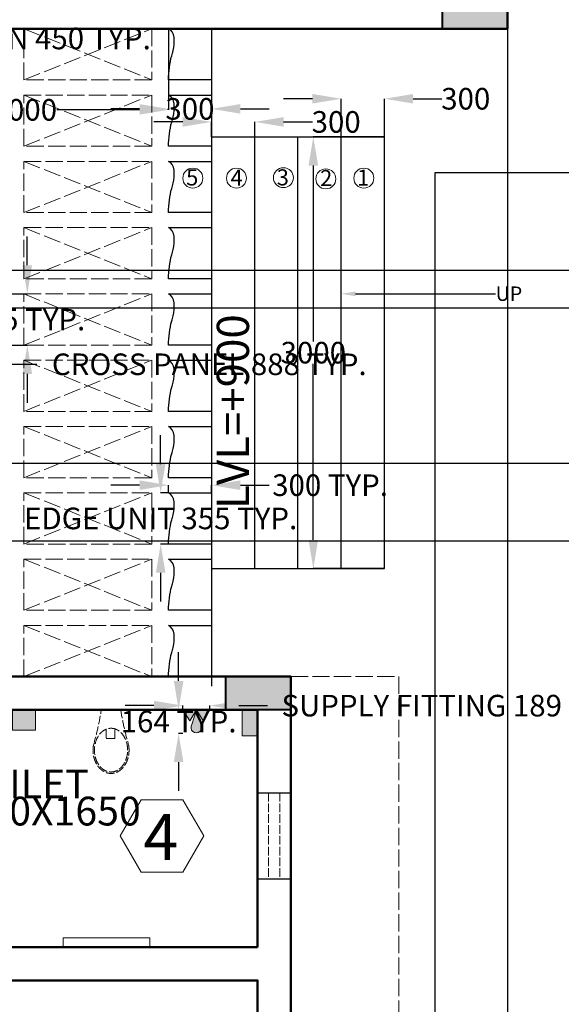
# Model space of a CAD drawing. Units: inches. Extents: x 22626 to 57351, y 2118 to 36234.
# Tile 7 of 10: x 45800 to 49561, y 16521 to 23360. Entities that reach past the tile are written whole.
import ezdxf
from ezdxf import colors
from ezdxf.entities.mleader import LeaderData, LeaderLine
from ezdxf.math import Vec2, Vec3

# ---------------------------------------------------------------- set-up
doc = ezdxf.new("R2010")
doc.units = ezdxf.units.IN
doc.header["$MEASUREMENT"] = 0
doc.linetypes.add('ACAD_ISO02W100', pattern=[15, 12, -3])
for name, color, linetype, lineweight in [('A-ANNO-DIMS', 130, 'Continuous', 18), ('A-ANNO-STRS', 130, 'Continuous', 15), ('A-ANNO-SYMB', 130, 'Continuous', 18), ('A-AREA-IDEN', 130, 'Continuous', 18), ('A-COLS', 7, 'Continuous', 40), ('A-FLOR-FIXT', 30, 'Continuous', 18), ('A-FLOR-FIXT-HIDN', 30, 'ACAD_ISO02W100', 18), ('A-GLAZ-VENT', 152, 'Continuous', 25), ('A-GLAZ-VENT-HIDN', 152, 'ACAD_ISO02W100', 18), ('A-ROOF', 80, 'Continuous', 25), ('A-ROOF-OVHD', 80, 'ACAD_ISO02W100', 18), ('A-WALL', 80, 'Continuous', 50), ('STAIRS', 82, 'Continuous', 25)]:
    doc.layers.add(name, color=color, linetype=linetype, lineweight=lineweight)
doc.styles.get("Standard").update_dxf_attribs({"font": 'arial.ttf'})
doc.dimstyles.get("Standard").update_dxf_attribs({"dimtxt": 150, "dimasz": 200, "dimexe": 0.18, "dimexo": 0.0625, "dimgap": 0.09, "dimtad": 0, "dimtih": 1, "dimtoh": 1, "dimdec": 0, "dimzin": 0, "dimdsep": 46, "dimtxsty": 'Standard', "dimcen": 0.09, "dimadec": 0, "dimazin": 0, "dimtfac": 1, "dimtdec": 0, "dimtofl": 0, "dimtmove": 0, "dimatfit": 3, "dimfxl": 1, "dimtolj": 1, "dimtzin": 0, "dimarcsym": 0})

# ---------------------------------------------------------------- blocks, each defined once
blk = doc.blocks.new('*D8')
at = {"layer": 'A-ANNO-DIMS', "color": 0, "lineweight": -2, "transparency": 16777216}
for p, q in [((48332.36654395866, 22546.86010836474), (47839.05636231795, 22546.86010836474)), ((47839.23636231794, 22346.86010836474), (47839.23636231794, 21123.587216141)), ((47839.23636231794, 19746.86010836474), (47839.23636231794, 20970.13300058848)), ((48332.36654395866, 19546.86010836473), (47839.05636231795, 19546.86010836473))]:
    blk.add_line(p, q, dxfattribs=at)
at = {"layer": 'A-ANNO-DIMS', "color": 0, "transparency": 16777216}
for points in [[(47805.90302898461, 22346.86010836474), (47872.56969565128, 22346.86010836474), (47839.23636231794, 22546.86010836474)], [(47805.90302898461, 19746.86010836474), (47872.56969565128, 19746.86010836474), (47839.23636231794, 19546.86010836473)]]:
    blk.add_solid(points, dxfattribs=at)
at = {"layer": 'Defpoints', "color": 0, "transparency": 16777216}
for p in [(48332.42904395866, 22546.86010836474), (47839.23636231794, 19546.86010836473), (48332.42904395866, 19546.86010836473)]:
    blk.add_point(p, dxfattribs=at)
at = {"layer": 'A-ANNO-DIMS', "color": 0, "transparency": 16777216, "insert": (47839.23636231794, 21046.86010836472), "char_height": 150, "attachment_point": 5}
blk.add_mtext('\\A1;3000', dxfattribs=at)
blk = doc.blocks.new('*D12')
at = {"layer": 'A-ANNO-DIMS', "color": 0, "lineweight": -2, "transparency": 16777216}
for p, q in [((44832.42904395864, 23296.79760836473), (44832.42904395864, 22733.54615739681)), ((46832.42904395864, 23296.79760836473), (46832.42904395864, 22733.54615739681)), ((45032.42904395865, 22733.72615739681), (45607.33904395865, 22733.72615739681)), ((46632.42904395865, 22733.72615739681), (46057.51904395864, 22733.72615739681))]:
    blk.add_line(p, q, dxfattribs=at)
at = {"layer": 'A-ANNO-DIMS', "color": 0, "transparency": 16777216}
for points in [[(45032.42904395865, 22767.05949073014), (45032.42904395865, 22700.39282406347), (44832.42904395864, 22733.72615739681)], [(46632.42904395865, 22767.05949073014), (46632.42904395865, 22700.39282406347), (46832.42904395864, 22733.72615739681)]]:
    blk.add_solid(points, dxfattribs=at)
at = {"layer": 'Defpoints', "color": 0, "transparency": 16777216}
for p in [(44832.42904395864, 23296.86010836473), (46832.42904395864, 23296.86010836473), (44832.42904395864, 22733.72615739681)]:
    blk.add_point(p, dxfattribs=at)
at = {"layer": 'A-ANNO-DIMS', "color": 0, "transparency": 16777216, "insert": (45832.42904395865, 22733.72615739681), "char_height": 150, "attachment_point": 5}
blk.add_mtext('\\A1;2000', dxfattribs=at)
blk = doc.blocks.new('*D13')
at = {"layer": 'A-ANNO-DIMS', "color": 0, "lineweight": -2, "transparency": 16777216}
for p, q in [((46632.22904395864, 22740.4612685317), (46432.22904395864, 22740.4612685317)), ((46832.22904395864, 22733.4086573968), (46832.22904395864, 22740.6412685317)), ((47132.42904395865, 22733.4086573968), (47132.42904395865, 22740.6412685317)), ((47332.42904395864, 22740.4612685317), (47532.42904395865, 22740.4612685317))]:
    blk.add_line(p, q, dxfattribs=at)
at = {"layer": 'A-ANNO-DIMS', "color": 0, "transparency": 16777216}
for points in [[(46632.22904395864, 22773.79460186503), (46632.22904395864, 22707.12793519837), (46832.22904395864, 22740.4612685317)], [(47332.42904395864, 22773.79460186503), (47332.42904395864, 22707.12793519837), (47132.42904395865, 22740.4612685317)]]:
    blk.add_solid(points, dxfattribs=at)
at = {"layer": 'Defpoints', "color": 0, "transparency": 16777216}
for p in [(46832.22904395864, 22733.34615739681), (47132.42904395865, 22740.4612685317), (47132.42904395865, 22733.34615739681)]:
    blk.add_point(p, dxfattribs=at)
at = {"layer": 'A-ANNO-DIMS', "color": 0, "transparency": 16777216, "insert": (46982.32904395864, 22740.4612685317), "char_height": 150, "attachment_point": 5}
blk.add_mtext('\\A1;300', dxfattribs=at)
blk = doc.blocks.new('*D14')
at = {"layer": 'A-ANNO-DIMS', "color": 0, "lineweight": -2, "transparency": 16777216}
for p, q in [((46932.42904395864, 22649.83293153023), (46732.42904395864, 22649.83293153023)), ((47132.42904395865, 22546.92260836473), (47132.42904395865, 22650.01293153023)), ((47432.42904395865, 22546.92260836473), (47432.42904395865, 22650.01293153023)), ((47632.42904395864, 22649.83293153023), (47832.42904395865, 22649.83293153023))]:
    blk.add_line(p, q, dxfattribs=at)
at = {"layer": 'A-ANNO-DIMS', "color": 0, "transparency": 16777216}
for points in [[(46932.42904395864, 22683.16626486356), (46932.42904395864, 22616.49959819689), (47132.42904395865, 22649.83293153023)], [(47632.42904395864, 22683.16626486356), (47632.42904395864, 22616.49959819689), (47432.42904395865, 22649.83293153023)]]:
    blk.add_solid(points, dxfattribs=at)
at = {"layer": 'Defpoints', "color": 0, "transparency": 16777216}
for p in [(47432.42904395865, 22649.83293153023), (47132.42904395865, 22546.86010836473), (47432.42904395865, 22546.86010836473)]:
    blk.add_point(p, dxfattribs=at)
at = {"layer": 'A-ANNO-DIMS', "color": 0, "transparency": 16777216, "insert": (47997.91808897911, 22649.83293153023), "char_height": 150, "attachment_point": 5}
blk.add_mtext('\\A1;300', dxfattribs=at)
blk = doc.blocks.new('*D15')
at = {"layer": 'A-ANNO-DIMS', "color": 0, "lineweight": -2, "transparency": 16777216}
for p, q in [((47832.42904395865, 22810.73997100012), (47632.42904395864, 22810.73997100012)), ((48032.42904395864, 22546.92260836473), (48032.42904395864, 22810.91997100012)), ((48332.42904395865, 22546.92260836473), (48332.42904395865, 22810.91997100012)), ((48532.42904395864, 22810.73997100012), (48732.42904395865, 22810.73997100012))]:
    blk.add_line(p, q, dxfattribs=at)
at = {"layer": 'A-ANNO-DIMS', "color": 0, "transparency": 16777216}
for points in [[(47832.42904395865, 22844.07330433345), (47832.42904395865, 22777.40663766679), (48032.42904395864, 22810.73997100012)], [(48532.42904395864, 22844.07330433345), (48532.42904395864, 22777.40663766679), (48332.42904395865, 22810.73997100012)]]:
    blk.add_solid(points, dxfattribs=at)
at = {"layer": 'Defpoints', "color": 0, "transparency": 16777216}
for p in [(48332.42904395865, 22810.73997100012), (48032.42904395864, 22546.86010836473), (48332.42904395865, 22546.86010836473)]:
    blk.add_point(p, dxfattribs=at)
at = {"layer": 'A-ANNO-DIMS', "color": 0, "transparency": 16777216, "insert": (48897.91808897911, 22810.73997100012), "char_height": 150, "attachment_point": 5}
blk.add_mtext('\\A1;300', dxfattribs=at)
blk = doc.blocks.new('WC')
at = {"ltscale": 5}
for p, q in [((307.4540408789253, 157.9229967620813), (242.2174300020561, 157.9229967620813)), ((242.2174300020561, 157.9229967620813), (242.2174300020561, 97.87988847275483)), ((307.4540408789253, 157.9229967620813), (307.4540408789253, 157.9229967620813)), ((242.2174300020561, 97.87988847275483), (310.0842174796853, 99.70460823710528))]:
    blk.add_line(p, q, dxfattribs=at)
for centre, start, end in [((780.732508801062, 2286.288249576111), 254.000576969056, 260.8285458946419), ((780.732508801062, -2036.267674000785), 99.17145410535805, 105.999423030944)]:
    blk.add_arc(centre, 2121.236142909723, start, end, dxfattribs=at)
blk.add_ellipse((161.9027973060947, 125.0102877876634), major_axis=(151.9040759523413, 0), ratio=0.7571275708385353, start_param=-1.570796326794896, end_param=4.712388980384689, dxfattribs=at)
for points, knots in [([(196.0611207178517, 247.2193096078299), (189.9898489161132, 248.2266596507652), (183.8456655129121, 248.9650412442752), (168.6182293347155, 250.1102459839712), (159.4964975931143, 250.2034131541222), (141.3581357193834, 249.212698022955), (132.3417047420516, 248.1288311957833), (114.6613914742556, 244.8098406800164), (105.9976853845146, 242.5747636017513), (89.26201623554518, 237.0062334978611), (81.19018288652298, 233.6728365616509), (65.86452451616788, 225.9859897466813), (58.61077128878969, 221.6325587335632), (45.13156838521536, 212.0080719868456), (38.90616664764093, 206.7369257869286), (27.67640637096338, 195.4043234284545), (22.67220516936504, 189.3426231032536), (14.05759261523781, 176.5860631599644), (10.44766267286468, 169.8909471035294), (4.765577569938614, 156.0629077761186), (2.69424158098991, 148.9301527436837), (0.1846293913040426, 134.463597005164), (-0.2530317139462568, 127.1307025187488), (0.5271766823570943, 112.5265070110981), (1.744832412616233, 105.2563518462193), (5.77749157987273, 91.03263116568269), (8.591685077881264, 84.07962673572185), (15.69573821845551, 70.70922901844096), (19.98490811580268, 64.29173781119243), (29.87879523489392, 52.16900764399179), (35.483208879421, 46.46348057011346), (47.82439502190391, 35.90657261581146), (54.56108629030495, 31.05501885116246), (68.96556532807881, 22.32099587028279), (76.63330319123634, 18.43849746629348), (92.68186228567357, 11.73355477496807), (101.0625846676266, 8.91115468616772), (118.3043576900527, 4.392898517646244), (127.1652540279829, 2.697098106120392), (144.6597339432555, 0.5298149587142689), (153.2812269904534, -0.000476238605188), (161.9027973060947, -0.000476238605188)], [1.35503494441986, 1.35503494441986, 1.35503494441986, 1.35503494441986, 1.471789532681877, 1.471789532681877, 1.642812487519809, 1.642812487519809, 1.813835442357741, 1.813835442357741, 1.984858397195673, 1.984858397195673, 2.155881352033606, 2.155881352033606, 2.326904306871538, 2.326904306871538, 2.49792726170947, 2.49792726170947, 2.668950216547402, 2.668950216547402, 2.839973171385334, 2.839973171385334, 3.010996126223266, 3.010996126223266, 3.182019081061198, 3.182019081061198, 3.35304203589913, 3.35304203589913, 3.524064990737062, 3.524064990737062, 3.695087945574994, 3.695087945574994, 3.866110900412926, 3.866110900412926, 4.037133855250859, 4.037133855250859, 4.208156810088791, 4.208156810088791, 4.379179764926723, 4.379179764926723, 4.550202719764655, 4.550202719764655, 4.712388980384689, 4.712388980384689, 4.712388980384689, 4.712388980384689]), ([(161.9027973060947, -0.000476238605188), (167.8851873344465, -0.000476238605188), (173.8675648995122, 0.254611844480678), (185.2699231324077, 1.230286525809788), (190.6953945214336, 1.911114408936555), (196.0639028232108, 2.802063691000512)], [-1.570796326794896, -1.570796326794896, -1.570796326794896, -1.570796326794896, -1.458257493061962, -1.458257493061962, -1.355016516099114, -1.355016516099114, -1.355016516099114, -1.355016516099114])]:
    blk.add_open_spline(points, degree=3, knots=knots, dxfattribs=at)
blk = doc.blocks.new('COL-RECTANGULAR')
h = blk.add_hatch(color=256)
h.dxf.hatch_style = 1
h.paths.add_polyline_path([(4.39586474386e-05, 0.0001083647293854), (450.0000439586474, 0.0001083647293854), (450.0000439586474, 230.0001083647294), (4.39586474386e-05, 230.0001083647294)])
blk.add_lwpolyline([(4.39586474386e-05, 0.0001083647293854), (4.39586474386e-05, 230.0001083647294), (450.0000439586474, 230.0001083647294), (450.0000439586474, 0.0001083647293854)], close=True)
blk = doc.blocks.new('CANOPY-CROSSED-PANEL')
at = {"ltscale": 10}
for p, q in [((4.39586510765e-05, -7.7958175098e-06), (887.5000439586511, 355.3241083647299)), ((4.39586510765e-05, 355.3241083647299), (887.5000439586511, -7.7958175098e-06))]:
    blk.add_line(p, q, dxfattribs=at)
blk.add_lwpolyline([(4.39586510765e-05, 355.3241083647299), (887.5000439586511, 355.3241083647299), (887.5000439586511, -7.7958175098e-06), (4.39586510765e-05, -7.7958175098e-06)], close=True, dxfattribs=at)
blk = doc.blocks.new('CANOPY-EDGE-UNIT')
blk.add_lwpolyline([(4.39586510765e-05, 355.3241083647299), (300.0000439586511, 355.3241083647299), (300.0000439586511, -7.7958211477e-06), (4.39586510765e-05, -7.7958211477e-06)])
blk.add_open_spline([(4.39586510765e-05, -7.7958211477e-06), (4.431511672410124, 57.50918677931622), (9.829222033331462, 127.5577565662788), (45.33431013918743, 237.7808474231315), (48.5081452225204, 340.4779943810172), (4.39586510765e-05, 355.3241083647299)], degree=3, knots=[0, 0, 0, 0, 169.2538425934583, 206.1581577034206, 361.8230239706648, 361.8230239706648, 361.8230239706648, 361.8230239706648])
blk = doc.blocks.new('BATH-SUPPLY-FITTING')
h = blk.add_hatch(color=256)
h.dxf.hatch_style = 1
h.paths.add_polyline_path([(161.0140439586466, 189.3806798614205), (84.84003036547074, 140.983449503361), (161.0140439586466, 94.69046873241678)])
h = blk.add_hatch(color=256)
h.dxf.hatch_style = 1
h.paths.add_polyline_path([(161.0140439586466, 94.69046873241678), (58.24591656582924, 125.2086534748123, 1.90856376211952), (58.24591656582924, 64.17228399002124)])
h = blk.add_hatch(color=256)
h.dxf.hatch_style = 1
h.paths.add_polyline_path([(161.0140439586466, 94.69046873241678), (84.84003036547074, 48.39748796147251), (161.0140439586466, 0.000257603413047)])
for p, q in [((161.0140439586466, 189.3806798614205), (84.84003036547074, 140.983449503361)), ((84.84003036547074, 140.983449503361), (161.0140439586466, 94.69046873241678)), ((161.0140439586466, 94.69046873241678), (58.24591656582924, 125.2086534748123)), ((161.0140439586466, 94.69046873241678), (58.24591656582924, 64.17228399002124)), ((84.84003036547074, 48.39748796147251), (161.0140439586466, 94.69046873241678)), ((161.0140439586466, 0.000257603413047), (84.84003036547074, 48.39748796147251))]:
    blk.add_line(p, q)
blk.add_arc((37.11803136635718, 94.69046873241678), 37.11801628553248, 55.30495923588778, 304.6950407641123)
blk = doc.blocks.new('BATH-WALL-ACCESSORY')
h = blk.add_hatch(color=256)
h.dxf.hatch_style = 1
h.paths.add_polyline_path([(142.8430439586445, 231.1050653827879), (71.42162994010141, 231.1050653827879), (71.42162994010141, 158.5160872540764), (81.4216299401014, 158.5160872540764), (81.42162994010869, 221.1050653827879), (142.8430439586445, 221.1050653827879)])
h = blk.add_hatch(color=256)
h.dxf.hatch_style = 1
h.paths.add_polyline_path([(142.8430439586445, 158.5160872540764), (0.0002159215582651, 158.5160872540764), (0.0002159215582651, -1.22242890939e-05), (142.8430439586445, -1.22242854559e-05)])
for p, q in [((71.42162994010141, 158.5160872540764), (71.42162994010141, 231.1050653827879)), ((71.42162994010141, 231.1050653827879), (142.8430439586445, 231.1050653827879)), ((81.42162994010869, 221.1050653827879), (142.8430439586445, 221.1050653827879)), ((81.4216299401014, 158.5160872540764), (81.42162994010869, 221.1050653827879)), ((142.8430439586445, 158.5160872540764), (0.0002159215582651, 158.5160872540764)), ((0.0002159215582651, 158.5160872540764), (0.0002159215582651, -1.22242890939e-05)), ((142.8430439586445, 158.5160872540764), (142.8430439586445, 158.5160872540764)), ((0.0002159215582651, -1.22242890939e-05), (142.8430439586445, -1.22242854559e-05))]:
    blk.add_line(p, q)
blk = doc.blocks.new('BATH-WALL-BOX')
h = blk.add_hatch(color=256)
h.dxf.hatch_style = 1
h.paths.add_polyline_path([(182.0210439586444, 106.8341357510071), (0.000183795193152, 106.8341357510071), (0.000183795193152, 0.0001083647293854), (182.0210439586444, 0.0001083647293854)])
for p, q in [((0.000183795193152, 0.0001083647293854), (0.000183795193152, 106.8341357510071)), ((0.000183795193152, 106.8341357510071), (182.0210439586444, 106.8341357510071)), ((182.0210439586444, 0.0001083647293854), (0.000183795193152, 0.0001083647293854))]:
    blk.add_line(p, q)
blk = doc.blocks.new('*D50')
at = {"layer": 'A-ANNO-DIMS', "color": 0, "lineweight": -2, "transparency": 16777216}
for p, q in [((44832.42904395864, 21099.39532160887), (44832.42904395864, 20966.15282160887)), ((45719.92904395863, 21099.39532160887), (45719.92904395863, 20966.15282160887)), ((45032.42904395864, 20966.33282160887), (45519.92904395864, 20966.33282160887)), ((45719.92904395863, 20966.33282160887), (45919.92904395864, 20966.33282160887))]:
    blk.add_line(p, q, dxfattribs=at)
at = {"layer": 'A-ANNO-DIMS', "color": 0, "transparency": 16777216}
for points in [[(45032.42904395864, 20999.6661549422), (45032.42904395864, 20932.99948827554), (44832.42904395864, 20966.33282160887)], [(45519.92904395864, 20999.6661549422), (45519.92904395864, 20932.99948827554), (45719.92904395863, 20966.33282160887)]]:
    blk.add_solid(points, dxfattribs=at)
at = {"layer": 'Defpoints', "color": 0, "transparency": 16777216}
for p in [(44832.42904395864, 21099.45782160887), (45719.92904395863, 21099.45782160887), (45719.92904395863, 20966.33282160887)]:
    blk.add_point(p, dxfattribs=at)
at = {"layer": 'A-ANNO-DIMS', "color": 0, "transparency": 16777216, "insert": (47116.89830726013, 20966.33282160887), "char_height": 150, "attachment_point": 5}
blk.add_mtext('\\A1;CROSS PANEL 888 TYP.', dxfattribs=at)
blk = doc.blocks.new('*D51')
at = {"layer": 'A-ANNO-DIMS', "color": 0, "lineweight": -2, "transparency": 16777216}
for p, q in [((45853.05404395866, 21654.78193776943), (45853.05404395866, 21854.78193776943)), ((45719.99154395865, 21454.78193776943), (45853.23404395866, 21454.78193776943)), ((45719.99154395865, 21099.45782160888), (45853.23404395866, 21099.45782160888)), ((45853.05404395866, 20899.45782160888), (45853.05404395866, 20699.45782160888))]:
    blk.add_line(p, q, dxfattribs=at)
at = {"layer": 'A-ANNO-DIMS', "color": 0, "transparency": 16777216}
for points in [[(45819.72071062534, 21654.78193776943), (45886.387377292, 21654.78193776943), (45853.05404395866, 21454.78193776943)], [(45819.72071062534, 20899.45782160888), (45886.387377292, 20899.45782160888), (45853.05404395866, 21099.45782160888)]]:
    blk.add_solid(points, dxfattribs=at)
at = {"layer": 'Defpoints', "color": 0, "transparency": 16777216}
for p in [(45719.92904395865, 21454.78193776943), (45853.05404395866, 21454.78193776943), (45719.92904395865, 21099.45782160888)]:
    blk.add_point(p, dxfattribs=at)
at = {"layer": 'A-ANNO-DIMS', "color": 0, "transparency": 16777216, "insert": (45853.05404395866, 21277.11987968914), "char_height": 150, "attachment_point": 5}
blk.add_mtext('\\A1;355 TYP.', dxfattribs=at)
blk = doc.blocks.new('*D54')
at = {"layer": 'A-ANNO-DIMS', "color": 0, "lineweight": -2, "transparency": 16777216}
for p, q in [((46779.13042653459, 20273.22330982295), (46779.13042653459, 20473.22330982295)), ((46832.36654395865, 20073.22330982295), (46778.95042653458, 20073.22330982295)), ((46832.36654395865, 19717.8991936624), (46778.95042653458, 19717.8991936624)), ((46779.13042653459, 19517.89919366239), (46779.13042653459, 19317.8991936624))]:
    blk.add_line(p, q, dxfattribs=at)
at = {"layer": 'A-ANNO-DIMS', "color": 0, "transparency": 16777216}
for points in [[(46745.79709320125, 20273.22330982295), (46812.46375986792, 20273.22330982295), (46779.13042653459, 20073.22330982295)], [(46745.79709320125, 19517.89919366239), (46812.46375986792, 19517.89919366239), (46779.13042653459, 19717.8991936624)]]:
    blk.add_solid(points, dxfattribs=at)
at = {"layer": 'Defpoints', "color": 0, "transparency": 16777216}
for p in [(46779.13042653459, 20073.22330982295), (46832.42904395865, 20073.22330982295), (46832.42904395865, 19717.8991936624)]:
    blk.add_point(p, dxfattribs=at)
at = {"layer": 'A-ANNO-DIMS', "color": 0, "transparency": 16777216, "insert": (46779.13042653459, 19895.56125174265), "char_height": 150, "attachment_point": 5}
blk.add_mtext('\\A1;EDGE UNIT 355 TYP.', dxfattribs=at)
blk = doc.blocks.new('*D55')
at = {"layer": 'A-ANNO-DIMS', "color": 0, "lineweight": -2, "transparency": 16777216}
for p, q in [((46632.42904395864, 20126.52192724702), (46432.42904395863, 20126.52192724702)), ((46832.42904395863, 20073.28580982294), (46832.42904395863, 20126.70192724702)), ((47132.42904395864, 20073.28580982294), (47132.42904395864, 20126.70192724702)), ((47332.42904395864, 20126.52192724702), (47532.42904395864, 20126.52192724702))]:
    blk.add_line(p, q, dxfattribs=at)
at = {"layer": 'A-ANNO-DIMS', "color": 0, "transparency": 16777216}
for points in [[(46632.42904395864, 20159.85526058035), (46632.42904395864, 20093.18859391369), (46832.42904395863, 20126.52192724702)], [(47332.42904395864, 20159.85526058035), (47332.42904395864, 20093.18859391369), (47132.42904395864, 20126.52192724702)]]:
    blk.add_solid(points, dxfattribs=at)
at = {"layer": 'Defpoints', "color": 0, "transparency": 16777216}
for p in [(47132.42904395864, 20126.52192724702), (46832.42904395863, 20073.22330982294), (47132.42904395864, 20073.22330982294)]:
    blk.add_point(p, dxfattribs=at)
at = {"layer": 'A-ANNO-DIMS', "color": 0, "transparency": 16777216, "insert": (47955.81372335837, 20126.52192724702), "char_height": 150, "attachment_point": 5}
blk.add_mtext('\\A1;300 TYP.', dxfattribs=at)
blk = doc.blocks.new('*D56')
at = {"layer": 'A-ANNO-DIMS', "color": 0, "lineweight": -2, "transparency": 16777216}
for p, q in [((44302.42904395863, 23296.79760836473), (44302.42904395863, 23229.18010836473)), ((44752.42904395862, 23296.79760836473), (44752.42904395862, 23229.18010836473)), ((44502.42904395863, 23229.36010836473), (44552.42904395862, 23229.36010836473)), ((44752.42904395862, 23229.36010836473), (44952.42904395862, 23229.36010836473))]:
    blk.add_line(p, q, dxfattribs=at)
at = {"layer": 'A-ANNO-DIMS', "color": 0, "transparency": 16777216}
for points in [[(44502.42904395863, 23262.69344169806), (44502.42904395863, 23196.0267750314), (44302.42904395863, 23229.36010836473)], [(44552.42904395862, 23262.69344169806), (44552.42904395862, 23196.0267750314), (44752.42904395862, 23229.36010836473)]]:
    blk.add_solid(points, dxfattribs=at)
at = {"layer": 'Defpoints', "color": 0, "transparency": 16777216}
for p in [(44302.42904395863, 23296.86010836473), (44752.42904395862, 23296.86010836473), (44752.42904395862, 23229.36010836473)]:
    blk.add_point(p, dxfattribs=at)
at = {"layer": 'A-ANNO-DIMS', "color": 0, "transparency": 16777216, "insert": (45858.14660193952, 23229.36010836473), "char_height": 150, "attachment_point": 5}
blk.add_mtext('\\A1;COLUMN 450 TYP.', dxfattribs=at)
blk = doc.blocks.new('*D66')
at = {"layer": 'A-ANNO-DIMS', "color": 0, "lineweight": -2, "transparency": 16777216}
for p, q in [((46732.21802730284, 18595.26717170344), (46532.21802730284, 18595.26717170344)), ((46932.21802730284, 18566.92260836473), (46932.21802730284, 18595.44717170344)), ((47121.59844956086, 18566.92260836473), (47121.59844956086, 18595.44717170344)), ((47321.59844956085, 18595.26717170344), (47521.59844956086, 18595.26717170344))]:
    blk.add_line(p, q, dxfattribs=at)
at = {"layer": 'A-ANNO-DIMS', "color": 0, "transparency": 16777216}
for points in [[(46732.21802730284, 18628.60050503677), (46732.21802730284, 18561.93383837011), (46932.21802730284, 18595.26717170344)], [(47321.59844956085, 18628.60050503677), (47321.59844956085, 18561.93383837011), (47121.59844956086, 18595.26717170344)]]:
    blk.add_solid(points, dxfattribs=at)
at = {"layer": 'Defpoints', "color": 0, "transparency": 16777216}
for p in [(46932.21802730284, 18566.86010836473), (47121.59844956086, 18595.26717170344), (47121.59844956086, 18566.86010836473)]:
    blk.add_point(p, dxfattribs=at)
at = {"layer": 'A-ANNO-DIMS', "color": 0, "transparency": 16777216, "insert": (48823.75188748719, 18595.26717170344), "char_height": 150, "attachment_point": 5}
blk.add_mtext('\\A1;SUPPLY FITTING 189 TYP.', dxfattribs=at)
blk = doc.blocks.new('*D67')
at = {"layer": 'A-ANNO-DIMS', "color": 0, "lineweight": -2, "transparency": 16777216}
for p, q in [((46903.81096396418, 18766.86010836474), (46903.81096396418, 18966.86010836474)), ((46932.15552730285, 18566.86010836474), (46903.63096396417, 18566.86010836474)), ((46932.15552730286, 18402.73068226325), (46903.63096396417, 18402.73068226325)), ((46903.81096396418, 18202.73068226325), (46903.81096396418, 18002.73068226325))]:
    blk.add_line(p, q, dxfattribs=at)
at = {"layer": 'A-ANNO-DIMS', "color": 0, "transparency": 16777216}
for points in [[(46870.47763063084, 18766.86010836474), (46937.14429729751, 18766.86010836474), (46903.81096396418, 18566.86010836474)], [(46870.47763063084, 18202.73068226325), (46937.14429729751, 18202.73068226325), (46903.81096396418, 18402.73068226325)]]:
    blk.add_solid(points, dxfattribs=at)
at = {"layer": 'Defpoints', "color": 0, "transparency": 16777216}
for p in [(46903.81096396418, 18566.86010836474), (46932.21802730286, 18566.86010836474), (46932.21802730286, 18402.73068226325)]:
    blk.add_point(p, dxfattribs=at)
at = {"layer": 'A-ANNO-DIMS', "color": 0, "transparency": 16777216, "insert": (46903.81096396418, 18484.79539531398), "char_height": 150, "attachment_point": 5}
blk.add_mtext('\\A1;164 TYP.', dxfattribs=at)
blk = doc.blocks.new('*D99')
at = {"layer": 'A-ANNO-DIMS', "color": 0, "lineweight": -2, "transparency": 16777216}
for p, q in [((41184.594559, 30456.86010800002), (57038.79342100006, 30456.86010800002)), ((57038.61342100005, 30256.86010800002), (57038.61342100005, 18933.58721577627)), ((57038.61342100006, 7456.860108000005), (57038.61342100005, 18780.13300022374)), ((43702.49154400001, 7256.860108000004), (57038.79342100006, 7256.860108000005))]:
    blk.add_line(p, q, dxfattribs=at)
at = {"layer": 'A-ANNO-DIMS', "color": 0, "transparency": 16777216}
for points in [[(57005.28008766672, 30256.86010800002), (57071.94675433339, 30256.86010800002), (57038.61342100005, 30456.86010800002)], [(57005.28008766673, 7456.860108000005), (57071.9467543334, 7456.860108000005), (57038.61342100006, 7256.860108000005)]]:
    blk.add_solid(points, dxfattribs=at)
at = {"layer": 'Defpoints', "color": 0, "transparency": 16777216}
for p in [(41184.53205900001, 30456.86010800002), (57038.61342100005, 30456.86010800002), (43702.42904400001, 7256.860108000004)]:
    blk.add_point(p, dxfattribs=at)
at = {"layer": 'A-ANNO-DIMS', "color": 0, "transparency": 16777216, "insert": (57038.61342100005, 18856.86010799999), "char_height": 150, "attachment_point": 5}
blk.add_mtext('\\A1;23200', dxfattribs=at)
blk = doc.blocks.new('*D100')
at = {"layer": 'A-ANNO-DIMS', "color": 0, "lineweight": -2, "transparency": 16777216}
for p, q in [((32057.429044, 23296.797608), (32057.429044, 2216.185148)), ((49187.429044, 23296.797608), (49187.429044, 2216.185148)), ((32257.429044, 2216.365148), (40347.407256824, 2216.365148)), ((48987.42904399999, 2216.365148), (40897.45083117598, 2216.365148))]:
    blk.add_line(p, q, dxfattribs=at)
at = {"layer": 'A-ANNO-DIMS', "color": 0, "transparency": 16777216}
for points in [[(32257.429044, 2249.698481333334), (32257.429044, 2183.031814666666), (32057.429044, 2216.365148)], [(48987.42904399999, 2249.698481333334), (48987.42904399999, 2183.031814666666), (49187.429044, 2216.365148)]]:
    blk.add_solid(points, dxfattribs=at)
at = {"layer": 'Defpoints', "color": 0, "transparency": 16777216}
for p in [(32057.429044, 23296.860108), (49187.429044, 23296.860108), (49187.429044, 2216.365148)]:
    blk.add_point(p, dxfattribs=at)
at = {"layer": 'A-ANNO-DIMS', "color": 0, "transparency": 16777216, "insert": (40622.42904399999, 2216.365148), "char_height": 150, "attachment_point": 5}
blk.add_mtext('\\A1;17130', dxfattribs=at)
blk = doc.blocks.new('*D103')
at = {"layer": 'A-ANNO-DIMS', "color": 0, "lineweight": -2, "transparency": 16777216}
for p, q in [((42815.80305500001, 21358.37110900001), (57038.79342100006, 21358.37110900001)), ((57038.61342100005, 21158.37110900001), (57038.61342100005, 20626.21988015826)), ((57038.61342100005, 19940.71675500001), (57038.61342100005, 20472.86798384176)), ((42815.80305500001, 19740.71675500001), (57038.79342100006, 19740.71675500001))]:
    blk.add_line(p, q, dxfattribs=at)
at = {"layer": 'A-ANNO-DIMS', "color": 0, "transparency": 16777216}
for points in [[(57005.28008766672, 21158.37110900001), (57071.94675433339, 21158.37110900001), (57038.61342100005, 21358.37110900001)], [(57005.28008766672, 19940.71675500001), (57071.94675433339, 19940.71675500001), (57038.61342100005, 19740.71675500001)]]:
    blk.add_solid(points, dxfattribs=at)
at = {"layer": 'Defpoints', "color": 0, "transparency": 16777216}
for p in [(42815.74055500001, 21358.37110900001), (57038.61342100005, 21358.37110900001), (42815.74055500001, 19740.71675500001)]:
    blk.add_point(p, dxfattribs=at)
at = {"layer": 'A-ANNO-DIMS', "color": 0, "transparency": 16777216, "insert": (57038.61342100005, 20549.54393199999), "char_height": 150, "attachment_point": 5}
blk.add_mtext('\\A1;1617.7', dxfattribs=at)
blk = doc.blocks.new('*D105')
at = {"layer": 'A-ANNO-DIMS', "color": 0, "lineweight": -2, "transparency": 16777216}
for p, q in [((39983.04002200002, 21620.08858600001), (57038.79342100006, 21620.08858600001)), ((57038.61342100005, 21420.08858600001), (57038.61342100005, 21026.96734327627)), ((57038.61342100005, 20480.39188500001), (57038.61342100005, 20873.51312772375)), ((39983.04002200002, 20280.39188500001), (57038.79342100006, 20280.39188500001))]:
    blk.add_line(p, q, dxfattribs=at)
at = {"layer": 'A-ANNO-DIMS', "color": 0, "transparency": 16777216}
for points in [[(57005.28008766672, 21420.08858600001), (57071.94675433339, 21420.08858600001), (57038.61342100005, 21620.08858600001)], [(57005.28008766672, 20480.39188500001), (57071.94675433339, 20480.39188500001), (57038.61342100005, 20280.39188500001)]]:
    blk.add_solid(points, dxfattribs=at)
at = {"layer": 'Defpoints', "color": 0, "transparency": 16777216}
for p in [(39982.97752200002, 21620.08858600001), (57038.61342100005, 21620.08858600001), (39982.97752200002, 20280.39188500001)]:
    blk.add_point(p, dxfattribs=at)
at = {"layer": 'A-ANNO-DIMS', "color": 0, "transparency": 16777216, "insert": (57038.61342100005, 20950.24023549999), "char_height": 150, "attachment_point": 5}
blk.add_mtext('\\A1;1339.7', dxfattribs=at)

msp = doc.modelspace()

# ---------------------------------------------------------------- linework, layer by layer
at = {"layer": 'A-ANNO-STRS'}
for centre in [(47002.73154709683, 22259.35932784166), (47305.55586349163, 22259.35932784166), (47631.69814518732, 22262.57939482488), (47926.0432495549, 22254.10602591401), (48190.01175202362, 22259.35932784166)]:
    msp.add_circle(centre, 69.28929435855127, dxfattribs=at)
at = {"layer": 'A-AREA-IDEN'}
msp.add_lwpolyline([(47079.24070318431, 17690.30695458368), (46934.03598919386, 17941.80889671364), (46643.626561213, 17941.80889671364), (46498.42184722255, 17690.30695458368), (46643.626561213, 17438.80501245374), (46934.03598919386, 17438.80501245374)], close=True, dxfattribs=at)
at = {"layer": 'A-FLOR-FIXT'}
msp.add_lwpolyline([(46103.10993695085, 16916.86010836473), (46705.01888059482, 16916.86010836473), (46705.01888059482, 16981.56653679588), (46103.10993695085, 16981.56653679588)], close=True, dxfattribs=at)
at = {"layer": 'A-GLAZ-VENT'}
msp.add_lwpolyline([(47452.33452353128, 17990.34814777121), (47682.33452353128, 17990.34814777121), (47682.52356438602, 17390.21632581241), (47452.52356438601, 17390.21632581241)], close=True, dxfattribs=at)
at = {"layer": 'A-GLAZ-VENT-HIDN', "ltscale": 5}
for p, q in [((47527.52356438602, 17990.34814777121), (47527.52356438602, 17390.21632581241)), ((47607.52356438602, 17990.34814777121), (47607.52356438602, 17390.21632581241))]:
    msp.add_line(p, q, dxfattribs=at)
at = {"layer": 'A-ROOF'}
msp.add_lwpolyline([(41184.53205853078, 30256.86010836474), (50187.42904395865, 30256.86010836473), (50187.42904395865, 25126.86010836473), (50187.42904395865, 22296.86010836473), (48682.42904395865, 22296.86010836473), (48682.42904395865, 11956.86010836473), (43702.42904395865, 11956.86010836473)], dxfattribs=at)
at = {"layer": 'A-ROOF-OVHD', "ltscale": 10}
for p, q in [((47682.42904395864, 18796.86010836473), (48432.42904395864, 18796.86010836473)), ((48432.42904395864, 18796.86010836473), (48432.42904395864, 12206.86010836474))]:
    msp.add_line(p, q, dxfattribs=at)
at = {"layer": 'A-WALL'}
for p, q in [((49187.42904395864, 25126.86010836473), (49187.42904395864, 23296.86010836473)), ((46457.42904395865, 23296.86010836473), (41227.42904395864, 23296.86010836473)), ((49187.42904395864, 23296.86010836473), (46457.42904395865, 23296.86010836473))]:
    msp.add_line(p, q, dxfattribs=at)
for points in [[(44302.42904395864, 16916.86010836473), (44302.42904395864, 18796.86010836473), (47682.42904395864, 18796.86010836473), (47682.42904395864, 16916.86010836473)], [(44532.42904395865, 16916.86010836473), (44532.42904395865, 18566.86010836473), (47452.42904395865, 18566.86010836473), (47452.42904395865, 16916.86010836473)], [(45427.40111056185, 16916.86010836473), (47452.42904395865, 16916.86010836473)], [(47682.42904395864, 16916.86010836473), (47682.42904395864, 12956.86010836473), (46352.42904395864, 12956.86010836473)], [(44415.49291284107, 13186.86010836469), (43252.42904395865, 13186.86010836473), (43252.42904395865, 16686.86010836473), (47452.42904395865, 16686.86010836473), (47452.42904395865, 13186.86010836473), (46352.42904395864, 13186.86010836473)]]:
    msp.add_lwpolyline(points, dxfattribs=at)
at = {"layer": 'STAIRS'}
for p, q in [((47132.42904395865, 22546.86010836473), (48332.42904395865, 22546.86010836473)), ((47432.42904395864, 19546.86010836473), (47432.42904395865, 22546.86010836473)), ((47732.42904395864, 19546.86010836473), (47732.42904395864, 22546.86010836473)), ((48032.42904395863, 19546.86010836473), (48032.42904395864, 22546.86010836473)), ((48332.42904395864, 19546.86010836473), (48332.42904395865, 22546.86010836473)), ((47132.42904395865, 19546.86010836473), (48332.42904395865, 19546.86010836473))]:
    msp.add_line(p, q, dxfattribs=at)
msp.add_lwpolyline([(47132.42904395865, 23231.01644955535), (47132.42904395865, 18731.01644955535)], dxfattribs=at)

# ---------------------------------------------------------------- block references
at = {"layer": 'A-COLS'}
for p in [(48737.42899999998, 23296.86), (47232.42899999998, 18566.86)]:
    msp.add_blockref('COL-RECTANGULAR', p, dxfattribs=at)
at = {"layer": 'A-FLOR-FIXT', "rotation": 90}
msp.add_blockref('BATH-WALL-ACCESSORY', (45909.32086860428, 18424.01706440608), dxfattribs=at)
at = {"layer": 'A-FLOR-FIXT', "extrusion": (0, 0, -1), "zscale": -1, "rotation": 90}
for name, p in [('BATH-SUPPLY-FITTING', (-46932.21776969943, 18405.84606440609)), ('BATH-WALL-BOX', (-47345.59490820764, 18384.83906440609))]:
    msp.add_blockref(name, p, dxfattribs=at)
at = {"layer": 'A-FLOR-FIXT-HIDN', "rotation": 90}
msp.add_blockref('WC', (46559.51003853091, 18124.23006440352), dxfattribs=at)
at = {"layer": 'A-ROOF'}
for p in [(46832.42899999999, 22941.536), (46832.42899999999, 22481.01645735117), (46832.42899999999, 22020.49691470234), (46832.42899999999, 21559.97737205352), (46832.42899999999, 21099.45782940469), (46832.42899999999, 20638.93828675586), (46832.42899999999, 20178.41874410704), (46832.42899999999, 19717.89920145821), (46832.42899999999, 19257.37965880938), (46832.42899999999, 18796.86011616055)]:
    msp.add_blockref('CANOPY-EDGE-UNIT', p, dxfattribs=at)
at = {"layer": 'A-ROOF-OVHD'}
for p in [(45829.79447419181, 22941.536), (45829.79447419181, 22481.01645735117), (45829.79447419181, 22020.49691470234), (45829.79447419181, 21559.97737205352), (45829.79447419181, 21099.45782940469), (45829.79447419181, 20638.93828675586), (45829.79447419181, 20178.41874410703), (45829.79447419181, 19717.8992014582), (45829.79447419181, 19257.37965880937), (45829.79447419181, 18796.86011616055)]:
    msp.add_blockref('CANOPY-CROSSED-PANEL', p, dxfattribs=at)

# ---------------------------------------------------------------- texts
at = {"layer": 'A-ANNO-STRS'}
for s, p in [('5', (46956.10760498492, 22208.23608862967)), ('4', (47264.5210258539, 22206.47585297066)), ('3', (47585.36686326801, 22209.08940806125)), ('2', (47886.55192998136, 22204.33044320757)), ('1', (48142.67772880546, 22207.02189435874))]:
    msp.add_text(s, height=111.3871373176516, dxfattribs=at).set_placement(p)
at = {"layer": 'A-ANNO-SYMB'}
msp.add_text('LVL=+900', height=223.5019622695094, rotation=90, dxfattribs=at).set_placement((47392.58904384932, 19961.25386117541))
at = {"layer": 'A-AREA-IDEN'}
for s, height, p in [('TOILET', 200, (45361.63687232576, 17951.24344582519)), ('2920X1650', 200, (45273.13660637152, 17762.78744241449)), ('4', 318.6677366595216, (46659.26888903533, 17523.6305494449))]:
    msp.add_text(s, height=height, dxfattribs=at).set_placement(p)

# ---------------------------------------------------------------- dimensions: what is measured, and where the dimension line sits
at = {"layer": 'A-ANNO-DIMS'}
for base, p1, p2, override, picture, middle in [((57038.61342100005, 30456.86010800002), (43702.42904399999, 7256.860107999999), (41184.53205899999, 30456.860108), {"dimdec": 0, "dimlfac": 1, "dimrnd": 0, "dimzin": 0, "dimdsep": 46, "dimlunit": 2}, '*D99', (57038.61342100005, 18856.86010799999)), ((57038.61342100005, 21620.08858600001), (39982.977522, 20280.391885), (39982.977522, 21620.088586), {"dimdec": 1, "dimlfac": 1, "dimrnd": 0, "dimzin": 0, "dimdsep": 46, "dimlunit": 2}, '*D105', (57038.61342100005, 20950.24023549999)), ((57038.61342100005, 21358.37110900001), (42815.740555, 19740.716755), (42815.740555, 21358.371109), {"dimdec": 1, "dimlfac": 1, "dimrnd": 0, "dimzin": 0, "dimdsep": 46, "dimlunit": 2}, '*D103', (57038.61342100005, 20549.54393199999))]:
    dim = msp.add_linear_dim(base=base, p1=p1, p2=p2, angle=90, dimstyle='Standard', override=override, dxfattribs=at)
    dim.commit()
    dim.dimension.update_dxf_attribs({"geometry": picture, "text_midpoint": middle})
for base, p1, p2, text, picture, middle in [((44752.42904395862, 23229.36010836473), (44302.42904395863, 23296.86010836473), (44752.42904395862, 23296.86010836473), 'COLUMN <> TYP.', '*D56', (45858.14660193952, 23229.36010836473)), ((45719.92904395863, 20966.33282160887), (44832.42904395864, 21099.45782160887), (45719.92904395863, 21099.45782160887), 'CROSS PANEL <> TYP.', '*D50', (47116.89830726013, 20966.33282160887)), ((47132.42904395864, 20126.52192724702), (46832.42904395863, 20073.22330982294), (47132.42904395864, 20073.22330982294), '<> TYP.', '*D55', (47955.81372335837, 20126.52192724702)), ((47121.59844956086, 18595.26717170344), (46932.21802730284, 18566.86010836473), (47121.59844956086, 18566.86010836473), 'SUPPLY FITTING <> TYP.', '*D66', (48823.75188748719, 18595.26717170344))]:
    dim = msp.add_linear_dim(base=base, p1=p1, p2=p2, text=text, dimstyle='Standard', override={"dimdec": 0, "dimlfac": 1, "dimrnd": 0, "dimzin": 0, "dimdsep": 46, "dimlunit": 2}, dxfattribs=at)
    dim.commit()
    dim.dimension.update_dxf_attribs({"geometry": picture, "text_midpoint": middle})
for base, p1, p2, override, picture, middle in [((49187.429044, 2216.365148), (32057.429044, 23296.860108), (49187.429044, 23296.860108), {"dimdec": 0, "dimlfac": 1, "dimrnd": 0, "dimzin": 0, "dimdsep": 46, "dimlunit": 2}, '*D100', (40622.42904399999, 2216.365148)), ((44832.42904395864, 22733.72615739681), (46832.42904395864, 23296.86010836473), (44832.42904395864, 23296.86010836473), {"dimclrd": 0, "dimclre": 0, "dimclrt": 0}, '*D12', (45832.42904395865, 22733.72615739681)), ((48332.42904395865, 22810.73997100012), (48032.42904395864, 22546.86010836473), (48332.42904395865, 22546.86010836473), {"dimclrd": 0, "dimclre": 0, "dimclrt": 0}, '*D15', (48897.91808897911, 22810.73997100012)), ((47432.42904395865, 22649.83293153023), (47132.42904395865, 22546.86010836473), (47432.42904395865, 22546.86010836473), {"dimclrd": 0, "dimclre": 0, "dimclrt": 0}, '*D14', (47997.91808897911, 22649.83293153023))]:
    dim = msp.add_linear_dim(base=base, p1=p1, p2=p2, dimstyle='Standard', override=override, dxfattribs=at)
    dim.commit()
    dim.dimension.update_dxf_attribs({"geometry": picture, "text_midpoint": middle})
dim = msp.add_linear_dim(base=(47132.42904395865, 22740.4612685317), p1=(46832.22904395864, 22733.34615739681), p2=(47132.42904395865, 22733.34615739681), dimstyle='Standard', override={"dimclrd": 0, "dimclre": 0, "dimclrt": 0}, dxfattribs=at)
dim.commit()
dim.dimension.update_dxf_attribs({"geometry": '*D13', "text_midpoint": (46982.32904395864, 22740.4612685317), "dimtype": 160})
dim = msp.add_linear_dim(base=(47839.23636231794, 19546.86010836473), p1=(48332.42904395865, 22546.86010836473), p2=(48332.42904395865, 19546.86010836473), angle=90, dimstyle='Standard', override={"dimclrd": 0, "dimclre": 0, "dimclrt": 0}, dxfattribs=at)
dim.commit()
dim.dimension.update_dxf_attribs({"geometry": '*D8', "text_midpoint": (47839.23636231794, 21046.86010836472), "dimtype": 160})
for base, p1, p2, angle, text, picture, middle in [((45853.05404395866, 21454.78193776943), (45719.92904395863, 21099.45782160887), (45719.92904395863, 21454.78193776942), 90, '<> TYP.', '*D51', (45853.05404395866, 21277.11987968914)), ((46779.13042653459, 20073.22330982295), (46832.42904395863, 19717.89919366239), (46832.42904395863, 20073.22330982294), 90, 'EDGE UNIT <> TYP.', '*D54', (46779.13042653459, 19895.56125174265)), ((46903.81096396418, 18566.86010836474), (46932.21802730285, 18402.73068226325), (46932.21802730284, 18566.86010836473), 90.00000000000254, '<> TYP.', '*D67', (46903.81096396418, 18484.79539531398))]:
    dim = msp.add_linear_dim(base=base, p1=p1, p2=p2, angle=angle, text=text, dimstyle='Standard', override={"dimdec": 0, "dimlfac": 1, "dimrnd": 0, "dimzin": 0, "dimdsep": 46, "dimlunit": 2}, dxfattribs=at)
    dim.commit()
    dim.dimension.update_dxf_attribs({"geometry": picture, "text_midpoint": middle})

# ---------------------------------------------------------------- leaders
at = {"layer": 'A-ANNO-STRS'}
ml = msp.add_multileader_mtext('Standard', dxfattribs=at)
ml.set_content('UP', color=256)
ml.set_leader_properties()
ml.build(insert=Vec2(0, 0))
ml.multileader.update_dxf_attribs({"dogleg_length": 0.36, "arrow_head_size": 100})
ctx = ml.context
ctx.base_point, ctx.char_height, ctx.arrow_head_size, ctx.landing_gap_size, ctx.plane_origin = Vec3(49105.15574117633, 21455.78782619661), 100, 100, 0.09, Vec3(49653.85525502224, 21455.78782619661)
notes = []
notes.append((ctx, [(0, (1, 1, 0), (49104.79574117633, 21455.78782619661), (1, 0), 0.36, [(0, [(48032.42904395864, 21455.78782619661)], 0, [])])]))
ctx.mtext.insert, ctx.mtext.flow_direction = Vec3(49105.24574117633, 21506.64048649675), 5
for ctx, leaders in notes:
    for number, flags, end, landing, length, lines in leaders:
        leader = LeaderData()
        leader.index, (leader.has_last_leader_line, leader.has_dogleg_vector, leader.attachment_direction) = number, flags
        leader.last_leader_point, leader.dogleg_vector, leader.dogleg_length = Vec3(end), Vec3(landing), length
        for number, points, colour, breaks in lines:
            line = LeaderLine()
            line.index, line.vertices, line.color, line.breaks = number, Vec3.list(points), colors.encode_raw_color(colour), breaks
            leader.lines.append(line)
        ctx.leaders.append(leader)

doc.saveas('drawing.dxf')
